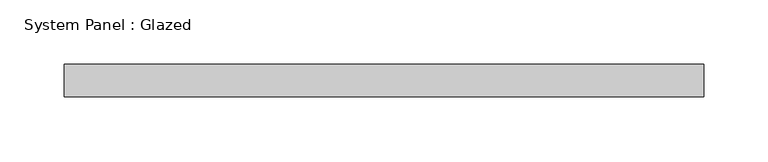
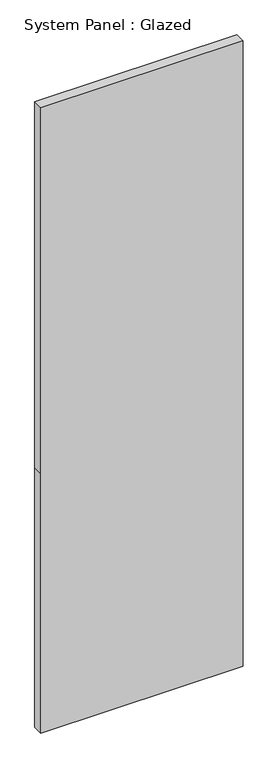
"""IFC4 building model written with IfcOpenShell, lengths in millimetres: plate geometry, System Panel : Glazed."""

from ifc_helpers import new_model, si_unit, frame, origin, place, context, project, spatial, polyline, outline, extrude, source, transform, mapped, element, save


def system_panel_glazed_0cc7d14b(model_context):
    return source(origin(), model_context, "Body", "SweptSolid", [
        extrude(outline(polyline([(0.0, -248.7083333), (0.0, 248.7083333), (673.1, 248.7083333), (1623.4675922, 248.7083333), (1623.4675922, -248.7083333), (673.1, -248.7083333), (0.0, -248.7083333)])), frame((0.0, 19.05, 0.0), z_axis=(0.0, 1.0, 0.0), x_axis=(0.0, 0.0, 1.0)), (0.0, 0.0, 1.0), 25.4),
    ])


if __name__ == "__main__":
    model = new_model("IFC4")
    model_context = context("Model", 3, world=origin())
    ifc_project = project(units=[si_unit("LENGTHUNIT", "METRE", prefix="MILLI")], contexts=[model_context])
    site = spatial("IfcSite", under=ifc_project)
    building = spatial("IfcBuilding", under=site)
    placement = place(None, origin())
    system_panel_glazed_shape = system_panel_glazed_0cc7d14b(model_context)
    element("IfcPlate", 1, ObjectType="System Panel : Glazed", at=placement, inside=building, context=model_context, shape_type="MappedRepresentation", body=[
        mapped(system_panel_glazed_shape, transform((0.0, 0.0, 0.0), x_axis=(1.0, 0.0, 0.0), y_axis=(0.0, 1.0, 0.0), z_axis=(0.0, 0.0, 1.0))),
    ])
    save(model, "model.ifc")

# Revit data of these elements
# Type "System Panel : Glazed"
#   Construction Type Id = "GSP4R"
#   Analytic Construction = "1/8 in Pilkington single glazing"
#   Visual Light Transmittance = 0.9
#   Solar Heat Gain Coefficient = 0.86
#   Heat Transfer Coefficient (U) = 1.18115 BTU/(h·ft²·°F)
#   Define Thermal Properties by = 1
# Element 1 (IfcPlate, "System Panel : Glazed")
#   Materials on its faces: "Glass"
# Materials
#   "Glass": class "Glass", colour RGB 0 128 192, transparency 0.75, Description = "Soda Lime Glass", Cost = 0
